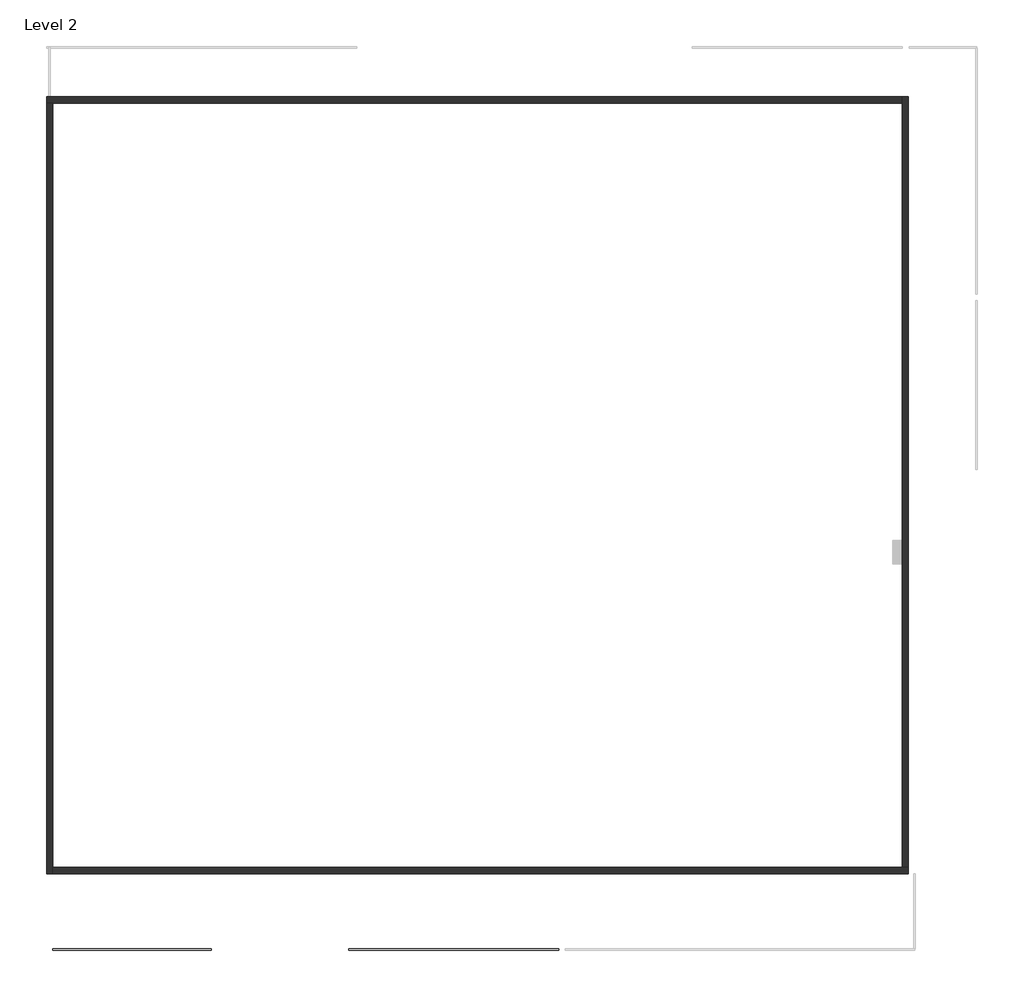
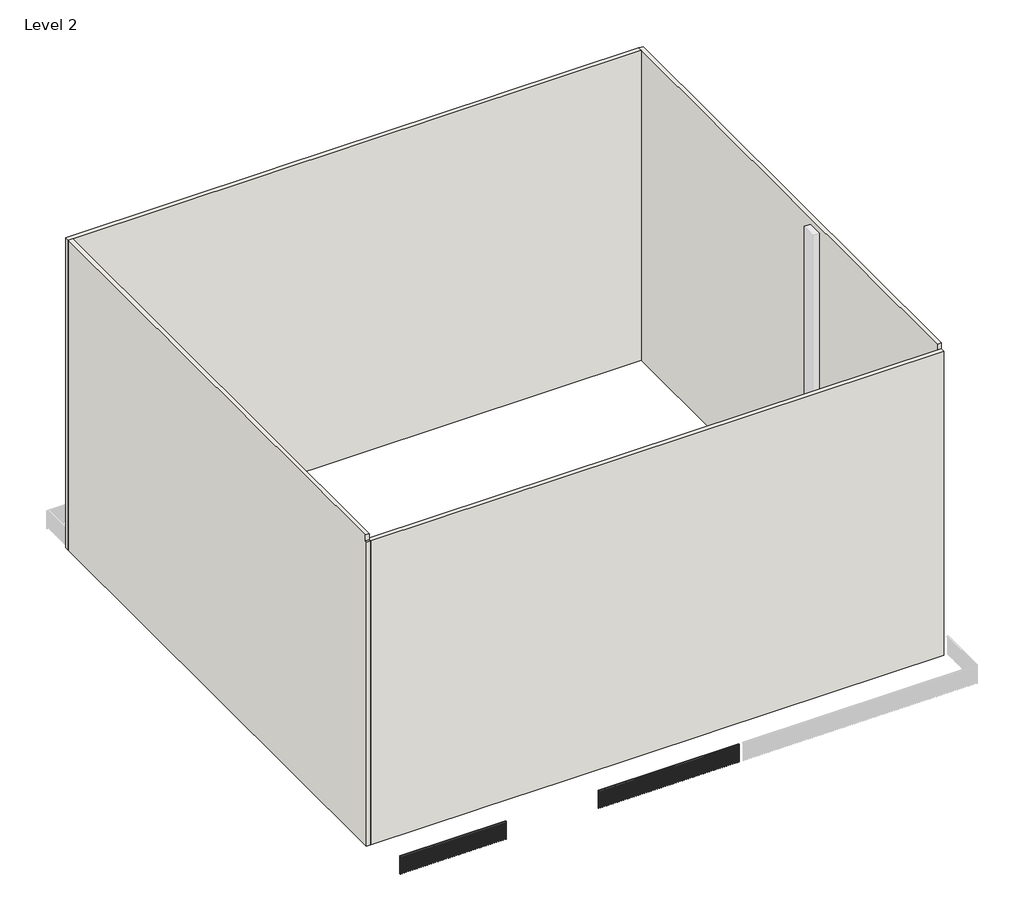
# One storey, part 1 of 5: 4 walls, 2 railings.
"""IFC4 building model written with IfcOpenShell, lengths in millimetres."""

from ifc_helpers import new_model, si_unit, frame, origin, place, context, project, spatial, polyline, outline, extrude, faceted_brep, element, save

model = new_model("IFC4")

# Units and contexts
model_context = context("Model", 3, world=origin())
ifc_project = project(units=[si_unit("LENGTHUNIT", "METRE", prefix="MILLI")], contexts=[model_context])

# Site, building, storey
site = spatial("IfcSite", under=ifc_project)
building = spatial("IfcBuilding", under=site)
storey = spatial("IfcBuildingStorey", under=building, Name="Level 2", Elevation=3048.0)

# Railings
placement = place(None, origin())
element("IfcRailing", 1, ObjectType="Handrail - Rectangular", at=placement, inside=storey, context=model_context, shape_type="SweptSolid", body=[
    extrude(outline(polyline([(-13630.2638778, -12911.7749501), (-13630.2638778, -12860.9749501), (-8499.4638778, -12860.9749501), (-8499.4638778, -12911.7749501), (-13630.2638778, -12911.7749501)])), frame((0.0, 0.0, 3911.6), z_axis=(0.0, 0.0, 1.0), x_axis=(1.0, 0.0, 0.0)), (0.0, 0.0, 1.0), 50.8),
    extrude(outline(polyline([(-8559.7888778, -12895.8999501), (-8559.7888778, -12876.8499501), (-8540.7388778, -12876.8499501), (-8540.7388778, -12895.8999501), (-8559.7888778, -12895.8999501)])), frame((0.0, 0.0, 3048.0), z_axis=(0.0, 0.0, 1.0), x_axis=(1.0, 0.0, 0.0)), (0.0, 0.0, 1.0), 863.6),
    extrude(outline(polyline([(-8661.3888778, -12895.8999501), (-8661.3888778, -12876.8499501), (-8642.3388778, -12876.8499501), (-8642.3388778, -12895.8999501), (-8661.3888778, -12895.8999501)])), frame((0.0, 0.0, 3048.0), z_axis=(0.0, 0.0, 1.0), x_axis=(1.0, 0.0, 0.0)), (0.0, 0.0, 1.0), 863.6),
    extrude(outline(polyline([(-8762.9888778, -12895.8999501), (-8762.9888778, -12876.8499501), (-8743.9388778, -12876.8499501), (-8743.9388778, -12895.8999501), (-8762.9888778, -12895.8999501)])), frame((0.0, 0.0, 3048.0), z_axis=(0.0, 0.0, 1.0), x_axis=(1.0, 0.0, 0.0)), (0.0, 0.0, 1.0), 863.6),
    extrude(outline(polyline([(-8864.5888778, -12895.8999501), (-8864.5888778, -12876.8499501), (-8845.5388778, -12876.8499501), (-8845.5388778, -12895.8999501), (-8864.5888778, -12895.8999501)])), frame((0.0, 0.0, 3048.0), z_axis=(0.0, 0.0, 1.0), x_axis=(1.0, 0.0, 0.0)), (0.0, 0.0, 1.0), 863.6),
    extrude(outline(polyline([(-8966.1888778, -12895.8999501), (-8966.1888778, -12876.8499501), (-8947.1388778, -12876.8499501), (-8947.1388778, -12895.8999501), (-8966.1888778, -12895.8999501)])), frame((0.0, 0.0, 3048.0), z_axis=(0.0, 0.0, 1.0), x_axis=(1.0, 0.0, 0.0)), (0.0, 0.0, 1.0), 863.6),
    extrude(outline(polyline([(-9067.7888778, -12895.8999501), (-9067.7888778, -12876.8499501), (-9048.7388778, -12876.8499501), (-9048.7388778, -12895.8999501), (-9067.7888778, -12895.8999501)])), frame((0.0, 0.0, 3048.0), z_axis=(0.0, 0.0, 1.0), x_axis=(1.0, 0.0, 0.0)), (0.0, 0.0, 1.0), 863.6),
    extrude(outline(polyline([(-9169.3888778, -12895.8999501), (-9169.3888778, -12876.8499501), (-9150.3388778, -12876.8499501), (-9150.3388778, -12895.8999501), (-9169.3888778, -12895.8999501)])), frame((0.0, 0.0, 3048.0), z_axis=(0.0, 0.0, 1.0), x_axis=(1.0, 0.0, 0.0)), (0.0, 0.0, 1.0), 863.6),
    extrude(outline(polyline([(-9270.9888778, -12895.8999501), (-9270.9888778, -12876.8499501), (-9251.9388778, -12876.8499501), (-9251.9388778, -12895.8999501), (-9270.9888778, -12895.8999501)])), frame((0.0, 0.0, 3048.0), z_axis=(0.0, 0.0, 1.0), x_axis=(1.0, 0.0, 0.0)), (0.0, 0.0, 1.0), 863.6),
    extrude(outline(polyline([(-9372.5888778, -12895.8999501), (-9372.5888778, -12876.8499501), (-9353.5388778, -12876.8499501), (-9353.5388778, -12895.8999501), (-9372.5888778, -12895.8999501)])), frame((0.0, 0.0, 3048.0), z_axis=(0.0, 0.0, 1.0), x_axis=(1.0, 0.0, 0.0)), (0.0, 0.0, 1.0), 863.6),
    extrude(outline(polyline([(-9474.1888778, -12895.8999501), (-9474.1888778, -12876.8499501), (-9455.1388778, -12876.8499501), (-9455.1388778, -12895.8999501), (-9474.1888778, -12895.8999501)])), frame((0.0, 0.0, 3048.0), z_axis=(0.0, 0.0, 1.0), x_axis=(1.0, 0.0, 0.0)), (0.0, 0.0, 1.0), 863.6),
    extrude(outline(polyline([(-9575.7888778, -12895.8999501), (-9575.7888778, -12876.8499501), (-9556.7388778, -12876.8499501), (-9556.7388778, -12895.8999501), (-9575.7888778, -12895.8999501)])), frame((0.0, 0.0, 3048.0), z_axis=(0.0, 0.0, 1.0), x_axis=(1.0, 0.0, 0.0)), (0.0, 0.0, 1.0), 863.6),
    extrude(outline(polyline([(-9677.3888778, -12895.8999501), (-9677.3888778, -12876.8499501), (-9658.3388778, -12876.8499501), (-9658.3388778, -12895.8999501), (-9677.3888778, -12895.8999501)])), frame((0.0, 0.0, 3048.0), z_axis=(0.0, 0.0, 1.0), x_axis=(1.0, 0.0, 0.0)), (0.0, 0.0, 1.0), 863.6),
    extrude(outline(polyline([(-9778.9888778, -12895.8999501), (-9778.9888778, -12876.8499501), (-9759.9388778, -12876.8499501), (-9759.9388778, -12895.8999501), (-9778.9888778, -12895.8999501)])), frame((0.0, 0.0, 3048.0), z_axis=(0.0, 0.0, 1.0), x_axis=(1.0, 0.0, 0.0)), (0.0, 0.0, 1.0), 863.6),
    extrude(outline(polyline([(-9880.5888778, -12895.8999501), (-9880.5888778, -12876.8499501), (-9861.5388778, -12876.8499501), (-9861.5388778, -12895.8999501), (-9880.5888778, -12895.8999501)])), frame((0.0, 0.0, 3048.0), z_axis=(0.0, 0.0, 1.0), x_axis=(1.0, 0.0, 0.0)), (0.0, 0.0, 1.0), 863.6),
    extrude(outline(polyline([(-9982.1888778, -12895.8999501), (-9982.1888778, -12876.8499501), (-9963.1388778, -12876.8499501), (-9963.1388778, -12895.8999501), (-9982.1888778, -12895.8999501)])), frame((0.0, 0.0, 3048.0), z_axis=(0.0, 0.0, 1.0), x_axis=(1.0, 0.0, 0.0)), (0.0, 0.0, 1.0), 863.6),
    extrude(outline(polyline([(-10083.7888778, -12895.8999501), (-10083.7888778, -12876.8499501), (-10064.7388778, -12876.8499501), (-10064.7388778, -12895.8999501), (-10083.7888778, -12895.8999501)])), frame((0.0, 0.0, 3048.0), z_axis=(0.0, 0.0, 1.0), x_axis=(1.0, 0.0, 0.0)), (0.0, 0.0, 1.0), 863.6),
    extrude(outline(polyline([(-10185.3888778, -12895.8999501), (-10185.3888778, -12876.8499501), (-10166.3388778, -12876.8499501), (-10166.3388778, -12895.8999501), (-10185.3888778, -12895.8999501)])), frame((0.0, 0.0, 3048.0), z_axis=(0.0, 0.0, 1.0), x_axis=(1.0, 0.0, 0.0)), (0.0, 0.0, 1.0), 863.6),
    extrude(outline(polyline([(-10286.9888778, -12895.8999501), (-10286.9888778, -12876.8499501), (-10267.9388778, -12876.8499501), (-10267.9388778, -12895.8999501), (-10286.9888778, -12895.8999501)])), frame((0.0, 0.0, 3048.0), z_axis=(0.0, 0.0, 1.0), x_axis=(1.0, 0.0, 0.0)), (0.0, 0.0, 1.0), 863.6),
    extrude(outline(polyline([(-10388.5888778, -12895.8999501), (-10388.5888778, -12876.8499501), (-10369.5388778, -12876.8499501), (-10369.5388778, -12895.8999501), (-10388.5888778, -12895.8999501)])), frame((0.0, 0.0, 3048.0), z_axis=(0.0, 0.0, 1.0), x_axis=(1.0, 0.0, 0.0)), (0.0, 0.0, 1.0), 863.6),
    extrude(outline(polyline([(-10490.1888778, -12895.8999501), (-10490.1888778, -12876.8499501), (-10471.1388778, -12876.8499501), (-10471.1388778, -12895.8999501), (-10490.1888778, -12895.8999501)])), frame((0.0, 0.0, 3048.0), z_axis=(0.0, 0.0, 1.0), x_axis=(1.0, 0.0, 0.0)), (0.0, 0.0, 1.0), 863.6),
    extrude(outline(polyline([(-10591.7888778, -12895.8999501), (-10591.7888778, -12876.8499501), (-10572.7388778, -12876.8499501), (-10572.7388778, -12895.8999501), (-10591.7888778, -12895.8999501)])), frame((0.0, 0.0, 3048.0), z_axis=(0.0, 0.0, 1.0), x_axis=(1.0, 0.0, 0.0)), (0.0, 0.0, 1.0), 863.6),
    extrude(outline(polyline([(-10693.3888778, -12895.8999501), (-10693.3888778, -12876.8499501), (-10674.3388778, -12876.8499501), (-10674.3388778, -12895.8999501), (-10693.3888778, -12895.8999501)])), frame((0.0, 0.0, 3048.0), z_axis=(0.0, 0.0, 1.0), x_axis=(1.0, 0.0, 0.0)), (0.0, 0.0, 1.0), 863.6),
    extrude(outline(polyline([(-10794.9888778, -12895.8999501), (-10794.9888778, -12876.8499501), (-10775.9388778, -12876.8499501), (-10775.9388778, -12895.8999501), (-10794.9888778, -12895.8999501)])), frame((0.0, 0.0, 3048.0), z_axis=(0.0, 0.0, 1.0), x_axis=(1.0, 0.0, 0.0)), (0.0, 0.0, 1.0), 863.6),
    extrude(outline(polyline([(-10896.5888778, -12895.8999501), (-10896.5888778, -12876.8499501), (-10877.5388778, -12876.8499501), (-10877.5388778, -12895.8999501), (-10896.5888778, -12895.8999501)])), frame((0.0, 0.0, 3048.0), z_axis=(0.0, 0.0, 1.0), x_axis=(1.0, 0.0, 0.0)), (0.0, 0.0, 1.0), 863.6),
    extrude(outline(polyline([(-10998.1888778, -12895.8999501), (-10998.1888778, -12876.8499501), (-10979.1388778, -12876.8499501), (-10979.1388778, -12895.8999501), (-10998.1888778, -12895.8999501)])), frame((0.0, 0.0, 3048.0), z_axis=(0.0, 0.0, 1.0), x_axis=(1.0, 0.0, 0.0)), (0.0, 0.0, 1.0), 863.6),
    extrude(outline(polyline([(-11099.7888778, -12895.8999501), (-11099.7888778, -12876.8499501), (-11080.7388778, -12876.8499501), (-11080.7388778, -12895.8999501), (-11099.7888778, -12895.8999501)])), frame((0.0, 0.0, 3048.0), z_axis=(0.0, 0.0, 1.0), x_axis=(1.0, 0.0, 0.0)), (0.0, 0.0, 1.0), 863.6),
    extrude(outline(polyline([(-11201.3888778, -12895.8999501), (-11201.3888778, -12876.8499501), (-11182.3388778, -12876.8499501), (-11182.3388778, -12895.8999501), (-11201.3888778, -12895.8999501)])), frame((0.0, 0.0, 3048.0), z_axis=(0.0, 0.0, 1.0), x_axis=(1.0, 0.0, 0.0)), (0.0, 0.0, 1.0), 863.6),
    extrude(outline(polyline([(-11302.9888778, -12895.8999501), (-11302.9888778, -12876.8499501), (-11283.9388778, -12876.8499501), (-11283.9388778, -12895.8999501), (-11302.9888778, -12895.8999501)])), frame((0.0, 0.0, 3048.0), z_axis=(0.0, 0.0, 1.0), x_axis=(1.0, 0.0, 0.0)), (0.0, 0.0, 1.0), 863.6),
    extrude(outline(polyline([(-11404.5888778, -12895.8999501), (-11404.5888778, -12876.8499501), (-11385.5388778, -12876.8499501), (-11385.5388778, -12895.8999501), (-11404.5888778, -12895.8999501)])), frame((0.0, 0.0, 3048.0), z_axis=(0.0, 0.0, 1.0), x_axis=(1.0, 0.0, 0.0)), (0.0, 0.0, 1.0), 863.6),
    extrude(outline(polyline([(-11506.1888778, -12895.8999501), (-11506.1888778, -12876.8499501), (-11487.1388778, -12876.8499501), (-11487.1388778, -12895.8999501), (-11506.1888778, -12895.8999501)])), frame((0.0, 0.0, 3048.0), z_axis=(0.0, 0.0, 1.0), x_axis=(1.0, 0.0, 0.0)), (0.0, 0.0, 1.0), 863.6),
    extrude(outline(polyline([(-11607.7888778, -12895.8999501), (-11607.7888778, -12876.8499501), (-11588.7388778, -12876.8499501), (-11588.7388778, -12895.8999501), (-11607.7888778, -12895.8999501)])), frame((0.0, 0.0, 3048.0), z_axis=(0.0, 0.0, 1.0), x_axis=(1.0, 0.0, 0.0)), (0.0, 0.0, 1.0), 863.6),
    extrude(outline(polyline([(-11709.3888778, -12895.8999501), (-11709.3888778, -12876.8499501), (-11690.3388778, -12876.8499501), (-11690.3388778, -12895.8999501), (-11709.3888778, -12895.8999501)])), frame((0.0, 0.0, 3048.0), z_axis=(0.0, 0.0, 1.0), x_axis=(1.0, 0.0, 0.0)), (0.0, 0.0, 1.0), 863.6),
    extrude(outline(polyline([(-11810.9888778, -12895.8999501), (-11810.9888778, -12876.8499501), (-11791.9388778, -12876.8499501), (-11791.9388778, -12895.8999501), (-11810.9888778, -12895.8999501)])), frame((0.0, 0.0, 3048.0), z_axis=(0.0, 0.0, 1.0), x_axis=(1.0, 0.0, 0.0)), (0.0, 0.0, 1.0), 863.6),
    extrude(outline(polyline([(-11912.5888778, -12895.8999501), (-11912.5888778, -12876.8499501), (-11893.5388778, -12876.8499501), (-11893.5388778, -12895.8999501), (-11912.5888778, -12895.8999501)])), frame((0.0, 0.0, 3048.0), z_axis=(0.0, 0.0, 1.0), x_axis=(1.0, 0.0, 0.0)), (0.0, 0.0, 1.0), 863.6),
    extrude(outline(polyline([(-12014.1888778, -12895.8999501), (-12014.1888778, -12876.8499501), (-11995.1388778, -12876.8499501), (-11995.1388778, -12895.8999501), (-12014.1888778, -12895.8999501)])), frame((0.0, 0.0, 3048.0), z_axis=(0.0, 0.0, 1.0), x_axis=(1.0, 0.0, 0.0)), (0.0, 0.0, 1.0), 863.6),
    extrude(outline(polyline([(-12115.7888778, -12895.8999501), (-12115.7888778, -12876.8499501), (-12096.7388778, -12876.8499501), (-12096.7388778, -12895.8999501), (-12115.7888778, -12895.8999501)])), frame((0.0, 0.0, 3048.0), z_axis=(0.0, 0.0, 1.0), x_axis=(1.0, 0.0, 0.0)), (0.0, 0.0, 1.0), 863.6),
    extrude(outline(polyline([(-12217.3888778, -12895.8999501), (-12217.3888778, -12876.8499501), (-12198.3388778, -12876.8499501), (-12198.3388778, -12895.8999501), (-12217.3888778, -12895.8999501)])), frame((0.0, 0.0, 3048.0), z_axis=(0.0, 0.0, 1.0), x_axis=(1.0, 0.0, 0.0)), (0.0, 0.0, 1.0), 863.6),
    extrude(outline(polyline([(-12318.9888778, -12895.8999501), (-12318.9888778, -12876.8499501), (-12299.9388778, -12876.8499501), (-12299.9388778, -12895.8999501), (-12318.9888778, -12895.8999501)])), frame((0.0, 0.0, 3048.0), z_axis=(0.0, 0.0, 1.0), x_axis=(1.0, 0.0, 0.0)), (0.0, 0.0, 1.0), 863.6),
    extrude(outline(polyline([(-12420.5888778, -12895.8999501), (-12420.5888778, -12876.8499501), (-12401.5388778, -12876.8499501), (-12401.5388778, -12895.8999501), (-12420.5888778, -12895.8999501)])), frame((0.0, 0.0, 3048.0), z_axis=(0.0, 0.0, 1.0), x_axis=(1.0, 0.0, 0.0)), (0.0, 0.0, 1.0), 863.6),
    extrude(outline(polyline([(-12522.1888778, -12895.8999501), (-12522.1888778, -12876.8499501), (-12503.1388778, -12876.8499501), (-12503.1388778, -12895.8999501), (-12522.1888778, -12895.8999501)])), frame((0.0, 0.0, 3048.0), z_axis=(0.0, 0.0, 1.0), x_axis=(1.0, 0.0, 0.0)), (0.0, 0.0, 1.0), 863.6),
    extrude(outline(polyline([(-12623.7888778, -12895.8999501), (-12623.7888778, -12876.8499501), (-12604.7388778, -12876.8499501), (-12604.7388778, -12895.8999501), (-12623.7888778, -12895.8999501)])), frame((0.0, 0.0, 3048.0), z_axis=(0.0, 0.0, 1.0), x_axis=(1.0, 0.0, 0.0)), (0.0, 0.0, 1.0), 863.6),
    extrude(outline(polyline([(-12725.3888778, -12895.8999501), (-12725.3888778, -12876.8499501), (-12706.3388778, -12876.8499501), (-12706.3388778, -12895.8999501), (-12725.3888778, -12895.8999501)])), frame((0.0, 0.0, 3048.0), z_axis=(0.0, 0.0, 1.0), x_axis=(1.0, 0.0, 0.0)), (0.0, 0.0, 1.0), 863.6),
    extrude(outline(polyline([(-12826.9888778, -12895.8999501), (-12826.9888778, -12876.8499501), (-12807.9388778, -12876.8499501), (-12807.9388778, -12895.8999501), (-12826.9888778, -12895.8999501)])), frame((0.0, 0.0, 3048.0), z_axis=(0.0, 0.0, 1.0), x_axis=(1.0, 0.0, 0.0)), (0.0, 0.0, 1.0), 863.6),
    extrude(outline(polyline([(-12928.5888778, -12895.8999501), (-12928.5888778, -12876.8499501), (-12909.5388778, -12876.8499501), (-12909.5388778, -12895.8999501), (-12928.5888778, -12895.8999501)])), frame((0.0, 0.0, 3048.0), z_axis=(0.0, 0.0, 1.0), x_axis=(1.0, 0.0, 0.0)), (0.0, 0.0, 1.0), 863.6),
    extrude(outline(polyline([(-13030.1888778, -12895.8999501), (-13030.1888778, -12876.8499501), (-13011.1388778, -12876.8499501), (-13011.1388778, -12895.8999501), (-13030.1888778, -12895.8999501)])), frame((0.0, 0.0, 3048.0), z_axis=(0.0, 0.0, 1.0), x_axis=(1.0, 0.0, 0.0)), (0.0, 0.0, 1.0), 863.6),
    extrude(outline(polyline([(-13131.7888778, -12895.8999501), (-13131.7888778, -12876.8499501), (-13112.7388778, -12876.8499501), (-13112.7388778, -12895.8999501), (-13131.7888778, -12895.8999501)])), frame((0.0, 0.0, 3048.0), z_axis=(0.0, 0.0, 1.0), x_axis=(1.0, 0.0, 0.0)), (0.0, 0.0, 1.0), 863.6),
    extrude(outline(polyline([(-13233.3888778, -12895.8999501), (-13233.3888778, -12876.8499501), (-13214.3388778, -12876.8499501), (-13214.3388778, -12895.8999501), (-13233.3888778, -12895.8999501)])), frame((0.0, 0.0, 3048.0), z_axis=(0.0, 0.0, 1.0), x_axis=(1.0, 0.0, 0.0)), (0.0, 0.0, 1.0), 863.6),
    extrude(outline(polyline([(-13334.9888778, -12895.8999501), (-13334.9888778, -12876.8499501), (-13315.9388778, -12876.8499501), (-13315.9388778, -12895.8999501), (-13334.9888778, -12895.8999501)])), frame((0.0, 0.0, 3048.0), z_axis=(0.0, 0.0, 1.0), x_axis=(1.0, 0.0, 0.0)), (0.0, 0.0, 1.0), 863.6),
    extrude(outline(polyline([(-13436.5888778, -12895.8999501), (-13436.5888778, -12876.8499501), (-13417.5388778, -12876.8499501), (-13417.5388778, -12895.8999501), (-13436.5888778, -12895.8999501)])), frame((0.0, 0.0, 3048.0), z_axis=(0.0, 0.0, 1.0), x_axis=(1.0, 0.0, 0.0)), (0.0, 0.0, 1.0), 863.6),
    extrude(outline(polyline([(-13538.1888778, -12895.8999501), (-13538.1888778, -12876.8499501), (-13519.1388778, -12876.8499501), (-13519.1388778, -12895.8999501), (-13538.1888778, -12895.8999501)])), frame((0.0, 0.0, 3048.0), z_axis=(0.0, 0.0, 1.0), x_axis=(1.0, 0.0, 0.0)), (0.0, 0.0, 1.0), 863.6),
    extrude(outline(polyline([(-8518.5138778, -12895.8999501), (-8518.5138778, -12876.8499501), (-8499.4638778, -12876.8499501), (-8499.4638778, -12895.8999501), (-8518.5138778, -12895.8999501)])), frame((0.0, 0.0, 3048.0), z_axis=(0.0, 0.0, 1.0), x_axis=(1.0, 0.0, 0.0)), (0.0, 0.0, 1.0), 863.6),
    extrude(outline(polyline([(-13630.2638778, -12895.8999501), (-13630.2638778, -12876.8499501), (-13611.2138778, -12876.8499501), (-13611.2138778, -12895.8999501), (-13630.2638778, -12895.8999501)])), frame((0.0, 0.0, 3048.0), z_axis=(0.0, 0.0, 1.0), x_axis=(1.0, 0.0, 0.0)), (0.0, 0.0, 1.0), 863.6),
])
element("IfcRailing", 2, ObjectType="Handrail - Rectangular", at=placement, inside=storey, context=model_context, shape_type="SweptSolid", body=[
    extrude(outline(polyline([(-4029.0638778, -12911.7749501), (-4029.0638778, -12860.9749501), (2778.1361222, -12860.9749501), (2778.1361222, -12911.7749501), (-4029.0638778, -12911.7749501)])), frame((0.0, 0.0, 3911.6), z_axis=(0.0, 0.0, 1.0), x_axis=(1.0, 0.0, 0.0)), (0.0, 0.0, 1.0), 50.8),
    extrude(outline(polyline([(2667.0111222, -12895.8999501), (2667.0111222, -12876.8499501), (2686.0611222, -12876.8499501), (2686.0611222, -12895.8999501), (2667.0111222, -12895.8999501)])), frame((0.0, 0.0, 3048.0), z_axis=(0.0, 0.0, 1.0), x_axis=(1.0, 0.0, 0.0)), (0.0, 0.0, 1.0), 863.6),
    extrude(outline(polyline([(2565.4111222, -12895.8999501), (2565.4111222, -12876.8499501), (2584.4611222, -12876.8499501), (2584.4611222, -12895.8999501), (2565.4111222, -12895.8999501)])), frame((0.0, 0.0, 3048.0), z_axis=(0.0, 0.0, 1.0), x_axis=(1.0, 0.0, 0.0)), (0.0, 0.0, 1.0), 863.6),
    extrude(outline(polyline([(2463.8111222, -12895.8999501), (2463.8111222, -12876.8499501), (2482.8611222, -12876.8499501), (2482.8611222, -12895.8999501), (2463.8111222, -12895.8999501)])), frame((0.0, 0.0, 3048.0), z_axis=(0.0, 0.0, 1.0), x_axis=(1.0, 0.0, 0.0)), (0.0, 0.0, 1.0), 863.6),
    extrude(outline(polyline([(2362.2111222, -12895.8999501), (2362.2111222, -12876.8499501), (2381.2611222, -12876.8499501), (2381.2611222, -12895.8999501), (2362.2111222, -12895.8999501)])), frame((0.0, 0.0, 3048.0), z_axis=(0.0, 0.0, 1.0), x_axis=(1.0, 0.0, 0.0)), (0.0, 0.0, 1.0), 863.6),
    extrude(outline(polyline([(2260.6111222, -12895.8999501), (2260.6111222, -12876.8499501), (2279.6611222, -12876.8499501), (2279.6611222, -12895.8999501), (2260.6111222, -12895.8999501)])), frame((0.0, 0.0, 3048.0), z_axis=(0.0, 0.0, 1.0), x_axis=(1.0, 0.0, 0.0)), (0.0, 0.0, 1.0), 863.6),
    extrude(outline(polyline([(2159.0111222, -12895.8999501), (2159.0111222, -12876.8499501), (2178.0611222, -12876.8499501), (2178.0611222, -12895.8999501), (2159.0111222, -12895.8999501)])), frame((0.0, 0.0, 3048.0), z_axis=(0.0, 0.0, 1.0), x_axis=(1.0, 0.0, 0.0)), (0.0, 0.0, 1.0), 863.6),
    extrude(outline(polyline([(2057.4111222, -12895.8999501), (2057.4111222, -12876.8499501), (2076.4611222, -12876.8499501), (2076.4611222, -12895.8999501), (2057.4111222, -12895.8999501)])), frame((0.0, 0.0, 3048.0), z_axis=(0.0, 0.0, 1.0), x_axis=(1.0, 0.0, 0.0)), (0.0, 0.0, 1.0), 863.6),
    extrude(outline(polyline([(1955.8111222, -12895.8999501), (1955.8111222, -12876.8499501), (1974.8611222, -12876.8499501), (1974.8611222, -12895.8999501), (1955.8111222, -12895.8999501)])), frame((0.0, 0.0, 3048.0), z_axis=(0.0, 0.0, 1.0), x_axis=(1.0, 0.0, 0.0)), (0.0, 0.0, 1.0), 863.6),
    extrude(outline(polyline([(1854.2111222, -12895.8999501), (1854.2111222, -12876.8499501), (1873.2611222, -12876.8499501), (1873.2611222, -12895.8999501), (1854.2111222, -12895.8999501)])), frame((0.0, 0.0, 3048.0), z_axis=(0.0, 0.0, 1.0), x_axis=(1.0, 0.0, 0.0)), (0.0, 0.0, 1.0), 863.6),
    extrude(outline(polyline([(1752.6111222, -12895.8999501), (1752.6111222, -12876.8499501), (1771.6611222, -12876.8499501), (1771.6611222, -12895.8999501), (1752.6111222, -12895.8999501)])), frame((0.0, 0.0, 3048.0), z_axis=(0.0, 0.0, 1.0), x_axis=(1.0, 0.0, 0.0)), (0.0, 0.0, 1.0), 863.6),
    extrude(outline(polyline([(1651.0111222, -12895.8999501), (1651.0111222, -12876.8499501), (1670.0611222, -12876.8499501), (1670.0611222, -12895.8999501), (1651.0111222, -12895.8999501)])), frame((0.0, 0.0, 3048.0), z_axis=(0.0, 0.0, 1.0), x_axis=(1.0, 0.0, 0.0)), (0.0, 0.0, 1.0), 863.6),
    extrude(outline(polyline([(1549.4111222, -12895.8999501), (1549.4111222, -12876.8499501), (1568.4611222, -12876.8499501), (1568.4611222, -12895.8999501), (1549.4111222, -12895.8999501)])), frame((0.0, 0.0, 3048.0), z_axis=(0.0, 0.0, 1.0), x_axis=(1.0, 0.0, 0.0)), (0.0, 0.0, 1.0), 863.6),
    extrude(outline(polyline([(1447.8111222, -12895.8999501), (1447.8111222, -12876.8499501), (1466.8611222, -12876.8499501), (1466.8611222, -12895.8999501), (1447.8111222, -12895.8999501)])), frame((0.0, 0.0, 3048.0), z_axis=(0.0, 0.0, 1.0), x_axis=(1.0, 0.0, 0.0)), (0.0, 0.0, 1.0), 863.6),
    extrude(outline(polyline([(1346.2111222, -12895.8999501), (1346.2111222, -12876.8499501), (1365.2611222, -12876.8499501), (1365.2611222, -12895.8999501), (1346.2111222, -12895.8999501)])), frame((0.0, 0.0, 3048.0), z_axis=(0.0, 0.0, 1.0), x_axis=(1.0, 0.0, 0.0)), (0.0, 0.0, 1.0), 863.6),
    extrude(outline(polyline([(1244.6111222, -12895.8999501), (1244.6111222, -12876.8499501), (1263.6611222, -12876.8499501), (1263.6611222, -12895.8999501), (1244.6111222, -12895.8999501)])), frame((0.0, 0.0, 3048.0), z_axis=(0.0, 0.0, 1.0), x_axis=(1.0, 0.0, 0.0)), (0.0, 0.0, 1.0), 863.6),
    extrude(outline(polyline([(1143.0111222, -12895.8999501), (1143.0111222, -12876.8499501), (1162.0611222, -12876.8499501), (1162.0611222, -12895.8999501), (1143.0111222, -12895.8999501)])), frame((0.0, 0.0, 3048.0), z_axis=(0.0, 0.0, 1.0), x_axis=(1.0, 0.0, 0.0)), (0.0, 0.0, 1.0), 863.6),
    extrude(outline(polyline([(1041.4111222, -12895.8999501), (1041.4111222, -12876.8499501), (1060.4611222, -12876.8499501), (1060.4611222, -12895.8999501), (1041.4111222, -12895.8999501)])), frame((0.0, 0.0, 3048.0), z_axis=(0.0, 0.0, 1.0), x_axis=(1.0, 0.0, 0.0)), (0.0, 0.0, 1.0), 863.6),
    extrude(outline(polyline([(939.8111222, -12895.8999501), (939.8111222, -12876.8499501), (958.8611222, -12876.8499501), (958.8611222, -12895.8999501), (939.8111222, -12895.8999501)])), frame((0.0, 0.0, 3048.0), z_axis=(0.0, 0.0, 1.0), x_axis=(1.0, 0.0, 0.0)), (0.0, 0.0, 1.0), 863.6),
    extrude(outline(polyline([(838.2111222, -12895.8999501), (838.2111222, -12876.8499501), (857.2611222, -12876.8499501), (857.2611222, -12895.8999501), (838.2111222, -12895.8999501)])), frame((0.0, 0.0, 3048.0), z_axis=(0.0, 0.0, 1.0), x_axis=(1.0, 0.0, 0.0)), (0.0, 0.0, 1.0), 863.6),
    extrude(outline(polyline([(736.6111222, -12895.8999501), (736.6111222, -12876.8499501), (755.6611222, -12876.8499501), (755.6611222, -12895.8999501), (736.6111222, -12895.8999501)])), frame((0.0, 0.0, 3048.0), z_axis=(0.0, 0.0, 1.0), x_axis=(1.0, 0.0, 0.0)), (0.0, 0.0, 1.0), 863.6),
    extrude(outline(polyline([(635.0111222, -12895.8999501), (635.0111222, -12876.8499501), (654.0611222, -12876.8499501), (654.0611222, -12895.8999501), (635.0111222, -12895.8999501)])), frame((0.0, 0.0, 3048.0), z_axis=(0.0, 0.0, 1.0), x_axis=(1.0, 0.0, 0.0)), (0.0, 0.0, 1.0), 863.6),
    extrude(outline(polyline([(533.4111222, -12895.8999501), (533.4111222, -12876.8499501), (552.4611222, -12876.8499501), (552.4611222, -12895.8999501), (533.4111222, -12895.8999501)])), frame((0.0, 0.0, 3048.0), z_axis=(0.0, 0.0, 1.0), x_axis=(1.0, 0.0, 0.0)), (0.0, 0.0, 1.0), 863.6),
    extrude(outline(polyline([(431.8111222, -12895.8999501), (431.8111222, -12876.8499501), (450.8611222, -12876.8499501), (450.8611222, -12895.8999501), (431.8111222, -12895.8999501)])), frame((0.0, 0.0, 3048.0), z_axis=(0.0, 0.0, 1.0), x_axis=(1.0, 0.0, 0.0)), (0.0, 0.0, 1.0), 863.6),
    extrude(outline(polyline([(330.2111222, -12895.8999501), (330.2111222, -12876.8499501), (349.2611222, -12876.8499501), (349.2611222, -12895.8999501), (330.2111222, -12895.8999501)])), frame((0.0, 0.0, 3048.0), z_axis=(0.0, 0.0, 1.0), x_axis=(1.0, 0.0, 0.0)), (0.0, 0.0, 1.0), 863.6),
    extrude(outline(polyline([(228.6111222, -12895.8999501), (228.6111222, -12876.8499501), (247.6611222, -12876.8499501), (247.6611222, -12895.8999501), (228.6111222, -12895.8999501)])), frame((0.0, 0.0, 3048.0), z_axis=(0.0, 0.0, 1.0), x_axis=(1.0, 0.0, 0.0)), (0.0, 0.0, 1.0), 863.6),
    extrude(outline(polyline([(127.0111222, -12895.8999501), (127.0111222, -12876.8499501), (146.0611222, -12876.8499501), (146.0611222, -12895.8999501), (127.0111222, -12895.8999501)])), frame((0.0, 0.0, 3048.0), z_axis=(0.0, 0.0, 1.0), x_axis=(1.0, 0.0, 0.0)), (0.0, 0.0, 1.0), 863.6),
    extrude(outline(polyline([(25.4111222, -12895.8999501), (25.4111222, -12876.8499501), (44.4611222, -12876.8499501), (44.4611222, -12895.8999501), (25.4111222, -12895.8999501)])), frame((0.0, 0.0, 3048.0), z_axis=(0.0, 0.0, 1.0), x_axis=(1.0, 0.0, 0.0)), (0.0, 0.0, 1.0), 863.6),
    extrude(outline(polyline([(-76.1888778, -12895.8999501), (-76.1888778, -12876.8499501), (-57.1388778, -12876.8499501), (-57.1388778, -12895.8999501), (-76.1888778, -12895.8999501)])), frame((0.0, 0.0, 3048.0), z_axis=(0.0, 0.0, 1.0), x_axis=(1.0, 0.0, 0.0)), (0.0, 0.0, 1.0), 863.6),
    extrude(outline(polyline([(-177.7888778, -12895.8999501), (-177.7888778, -12876.8499501), (-158.7388778, -12876.8499501), (-158.7388778, -12895.8999501), (-177.7888778, -12895.8999501)])), frame((0.0, 0.0, 3048.0), z_axis=(0.0, 0.0, 1.0), x_axis=(1.0, 0.0, 0.0)), (0.0, 0.0, 1.0), 863.6),
    extrude(outline(polyline([(-279.3888778, -12895.8999501), (-279.3888778, -12876.8499501), (-260.3388778, -12876.8499501), (-260.3388778, -12895.8999501), (-279.3888778, -12895.8999501)])), frame((0.0, 0.0, 3048.0), z_axis=(0.0, 0.0, 1.0), x_axis=(1.0, 0.0, 0.0)), (0.0, 0.0, 1.0), 863.6),
    extrude(outline(polyline([(-380.9888778, -12895.8999501), (-380.9888778, -12876.8499501), (-361.9388778, -12876.8499501), (-361.9388778, -12895.8999501), (-380.9888778, -12895.8999501)])), frame((0.0, 0.0, 3048.0), z_axis=(0.0, 0.0, 1.0), x_axis=(1.0, 0.0, 0.0)), (0.0, 0.0, 1.0), 863.6),
    extrude(outline(polyline([(-482.5888778, -12895.8999501), (-482.5888778, -12876.8499501), (-463.5388778, -12876.8499501), (-463.5388778, -12895.8999501), (-482.5888778, -12895.8999501)])), frame((0.0, 0.0, 3048.0), z_axis=(0.0, 0.0, 1.0), x_axis=(1.0, 0.0, 0.0)), (0.0, 0.0, 1.0), 863.6),
    extrude(outline(polyline([(-584.1888778, -12895.8999501), (-584.1888778, -12876.8499501), (-565.1388778, -12876.8499501), (-565.1388778, -12895.8999501), (-584.1888778, -12895.8999501)])), frame((0.0, 0.0, 3048.0), z_axis=(0.0, 0.0, 1.0), x_axis=(1.0, 0.0, 0.0)), (0.0, 0.0, 1.0), 863.6),
    extrude(outline(polyline([(-685.7888778, -12895.8999501), (-685.7888778, -12876.8499501), (-666.7388778, -12876.8499501), (-666.7388778, -12895.8999501), (-685.7888778, -12895.8999501)])), frame((0.0, 0.0, 3048.0), z_axis=(0.0, 0.0, 1.0), x_axis=(1.0, 0.0, 0.0)), (0.0, 0.0, 1.0), 863.6),
    extrude(outline(polyline([(-787.3888778, -12895.8999501), (-787.3888778, -12876.8499501), (-768.3388778, -12876.8499501), (-768.3388778, -12895.8999501), (-787.3888778, -12895.8999501)])), frame((0.0, 0.0, 3048.0), z_axis=(0.0, 0.0, 1.0), x_axis=(1.0, 0.0, 0.0)), (0.0, 0.0, 1.0), 863.6),
    extrude(outline(polyline([(-888.9888778, -12895.8999501), (-888.9888778, -12876.8499501), (-869.9388778, -12876.8499501), (-869.9388778, -12895.8999501), (-888.9888778, -12895.8999501)])), frame((0.0, 0.0, 3048.0), z_axis=(0.0, 0.0, 1.0), x_axis=(1.0, 0.0, 0.0)), (0.0, 0.0, 1.0), 863.6),
    extrude(outline(polyline([(-990.5888778, -12895.8999501), (-990.5888778, -12876.8499501), (-971.5388778, -12876.8499501), (-971.5388778, -12895.8999501), (-990.5888778, -12895.8999501)])), frame((0.0, 0.0, 3048.0), z_axis=(0.0, 0.0, 1.0), x_axis=(1.0, 0.0, 0.0)), (0.0, 0.0, 1.0), 863.6),
    extrude(outline(polyline([(-1092.1888778, -12895.8999501), (-1092.1888778, -12876.8499501), (-1073.1388778, -12876.8499501), (-1073.1388778, -12895.8999501), (-1092.1888778, -12895.8999501)])), frame((0.0, 0.0, 3048.0), z_axis=(0.0, 0.0, 1.0), x_axis=(1.0, 0.0, 0.0)), (0.0, 0.0, 1.0), 863.6),
    extrude(outline(polyline([(-1193.7888778, -12895.8999501), (-1193.7888778, -12876.8499501), (-1174.7388778, -12876.8499501), (-1174.7388778, -12895.8999501), (-1193.7888778, -12895.8999501)])), frame((0.0, 0.0, 3048.0), z_axis=(0.0, 0.0, 1.0), x_axis=(1.0, 0.0, 0.0)), (0.0, 0.0, 1.0), 863.6),
    extrude(outline(polyline([(-1295.3888778, -12895.8999501), (-1295.3888778, -12876.8499501), (-1276.3388778, -12876.8499501), (-1276.3388778, -12895.8999501), (-1295.3888778, -12895.8999501)])), frame((0.0, 0.0, 3048.0), z_axis=(0.0, 0.0, 1.0), x_axis=(1.0, 0.0, 0.0)), (0.0, 0.0, 1.0), 863.6),
    extrude(outline(polyline([(-1396.9888778, -12895.8999501), (-1396.9888778, -12876.8499501), (-1377.9388778, -12876.8499501), (-1377.9388778, -12895.8999501), (-1396.9888778, -12895.8999501)])), frame((0.0, 0.0, 3048.0), z_axis=(0.0, 0.0, 1.0), x_axis=(1.0, 0.0, 0.0)), (0.0, 0.0, 1.0), 863.6),
    extrude(outline(polyline([(-1498.5888778, -12895.8999501), (-1498.5888778, -12876.8499501), (-1479.5388778, -12876.8499501), (-1479.5388778, -12895.8999501), (-1498.5888778, -12895.8999501)])), frame((0.0, 0.0, 3048.0), z_axis=(0.0, 0.0, 1.0), x_axis=(1.0, 0.0, 0.0)), (0.0, 0.0, 1.0), 863.6),
    extrude(outline(polyline([(-1600.1888778, -12895.8999501), (-1600.1888778, -12876.8499501), (-1581.1388778, -12876.8499501), (-1581.1388778, -12895.8999501), (-1600.1888778, -12895.8999501)])), frame((0.0, 0.0, 3048.0), z_axis=(0.0, 0.0, 1.0), x_axis=(1.0, 0.0, 0.0)), (0.0, 0.0, 1.0), 863.6),
    extrude(outline(polyline([(-1701.7888778, -12895.8999501), (-1701.7888778, -12876.8499501), (-1682.7388778, -12876.8499501), (-1682.7388778, -12895.8999501), (-1701.7888778, -12895.8999501)])), frame((0.0, 0.0, 3048.0), z_axis=(0.0, 0.0, 1.0), x_axis=(1.0, 0.0, 0.0)), (0.0, 0.0, 1.0), 863.6),
    extrude(outline(polyline([(-1803.3888778, -12895.8999501), (-1803.3888778, -12876.8499501), (-1784.3388778, -12876.8499501), (-1784.3388778, -12895.8999501), (-1803.3888778, -12895.8999501)])), frame((0.0, 0.0, 3048.0), z_axis=(0.0, 0.0, 1.0), x_axis=(1.0, 0.0, 0.0)), (0.0, 0.0, 1.0), 863.6),
    extrude(outline(polyline([(-1904.9888778, -12895.8999501), (-1904.9888778, -12876.8499501), (-1885.9388778, -12876.8499501), (-1885.9388778, -12895.8999501), (-1904.9888778, -12895.8999501)])), frame((0.0, 0.0, 3048.0), z_axis=(0.0, 0.0, 1.0), x_axis=(1.0, 0.0, 0.0)), (0.0, 0.0, 1.0), 863.6),
    extrude(outline(polyline([(-2006.5888778, -12895.8999501), (-2006.5888778, -12876.8499501), (-1987.5388778, -12876.8499501), (-1987.5388778, -12895.8999501), (-2006.5888778, -12895.8999501)])), frame((0.0, 0.0, 3048.0), z_axis=(0.0, 0.0, 1.0), x_axis=(1.0, 0.0, 0.0)), (0.0, 0.0, 1.0), 863.6),
    extrude(outline(polyline([(-2108.1888778, -12895.8999501), (-2108.1888778, -12876.8499501), (-2089.1388778, -12876.8499501), (-2089.1388778, -12895.8999501), (-2108.1888778, -12895.8999501)])), frame((0.0, 0.0, 3048.0), z_axis=(0.0, 0.0, 1.0), x_axis=(1.0, 0.0, 0.0)), (0.0, 0.0, 1.0), 863.6),
    extrude(outline(polyline([(-2209.7888778, -12895.8999501), (-2209.7888778, -12876.8499501), (-2190.7388778, -12876.8499501), (-2190.7388778, -12895.8999501), (-2209.7888778, -12895.8999501)])), frame((0.0, 0.0, 3048.0), z_axis=(0.0, 0.0, 1.0), x_axis=(1.0, 0.0, 0.0)), (0.0, 0.0, 1.0), 863.6),
    extrude(outline(polyline([(-2311.3888778, -12895.8999501), (-2311.3888778, -12876.8499501), (-2292.3388778, -12876.8499501), (-2292.3388778, -12895.8999501), (-2311.3888778, -12895.8999501)])), frame((0.0, 0.0, 3048.0), z_axis=(0.0, 0.0, 1.0), x_axis=(1.0, 0.0, 0.0)), (0.0, 0.0, 1.0), 863.6),
    extrude(outline(polyline([(-2412.9888778, -12895.8999501), (-2412.9888778, -12876.8499501), (-2393.9388778, -12876.8499501), (-2393.9388778, -12895.8999501), (-2412.9888778, -12895.8999501)])), frame((0.0, 0.0, 3048.0), z_axis=(0.0, 0.0, 1.0), x_axis=(1.0, 0.0, 0.0)), (0.0, 0.0, 1.0), 863.6),
    extrude(outline(polyline([(-2514.5888778, -12895.8999501), (-2514.5888778, -12876.8499501), (-2495.5388778, -12876.8499501), (-2495.5388778, -12895.8999501), (-2514.5888778, -12895.8999501)])), frame((0.0, 0.0, 3048.0), z_axis=(0.0, 0.0, 1.0), x_axis=(1.0, 0.0, 0.0)), (0.0, 0.0, 1.0), 863.6),
    extrude(outline(polyline([(-2616.1888778, -12895.8999501), (-2616.1888778, -12876.8499501), (-2597.1388778, -12876.8499501), (-2597.1388778, -12895.8999501), (-2616.1888778, -12895.8999501)])), frame((0.0, 0.0, 3048.0), z_axis=(0.0, 0.0, 1.0), x_axis=(1.0, 0.0, 0.0)), (0.0, 0.0, 1.0), 863.6),
    extrude(outline(polyline([(-2717.7888778, -12895.8999501), (-2717.7888778, -12876.8499501), (-2698.7388778, -12876.8499501), (-2698.7388778, -12895.8999501), (-2717.7888778, -12895.8999501)])), frame((0.0, 0.0, 3048.0), z_axis=(0.0, 0.0, 1.0), x_axis=(1.0, 0.0, 0.0)), (0.0, 0.0, 1.0), 863.6),
    extrude(outline(polyline([(-2819.3888778, -12895.8999501), (-2819.3888778, -12876.8499501), (-2800.3388778, -12876.8499501), (-2800.3388778, -12895.8999501), (-2819.3888778, -12895.8999501)])), frame((0.0, 0.0, 3048.0), z_axis=(0.0, 0.0, 1.0), x_axis=(1.0, 0.0, 0.0)), (0.0, 0.0, 1.0), 863.6),
    extrude(outline(polyline([(-2920.9888778, -12895.8999501), (-2920.9888778, -12876.8499501), (-2901.9388778, -12876.8499501), (-2901.9388778, -12895.8999501), (-2920.9888778, -12895.8999501)])), frame((0.0, 0.0, 3048.0), z_axis=(0.0, 0.0, 1.0), x_axis=(1.0, 0.0, 0.0)), (0.0, 0.0, 1.0), 863.6),
    extrude(outline(polyline([(-3022.5888778, -12895.8999501), (-3022.5888778, -12876.8499501), (-3003.5388778, -12876.8499501), (-3003.5388778, -12895.8999501), (-3022.5888778, -12895.8999501)])), frame((0.0, 0.0, 3048.0), z_axis=(0.0, 0.0, 1.0), x_axis=(1.0, 0.0, 0.0)), (0.0, 0.0, 1.0), 863.6),
    extrude(outline(polyline([(-3124.1888778, -12895.8999501), (-3124.1888778, -12876.8499501), (-3105.1388778, -12876.8499501), (-3105.1388778, -12895.8999501), (-3124.1888778, -12895.8999501)])), frame((0.0, 0.0, 3048.0), z_axis=(0.0, 0.0, 1.0), x_axis=(1.0, 0.0, 0.0)), (0.0, 0.0, 1.0), 863.6),
    extrude(outline(polyline([(-3225.7888778, -12895.8999501), (-3225.7888778, -12876.8499501), (-3206.7388778, -12876.8499501), (-3206.7388778, -12895.8999501), (-3225.7888778, -12895.8999501)])), frame((0.0, 0.0, 3048.0), z_axis=(0.0, 0.0, 1.0), x_axis=(1.0, 0.0, 0.0)), (0.0, 0.0, 1.0), 863.6),
    extrude(outline(polyline([(-3327.3888778, -12895.8999501), (-3327.3888778, -12876.8499501), (-3308.3388778, -12876.8499501), (-3308.3388778, -12895.8999501), (-3327.3888778, -12895.8999501)])), frame((0.0, 0.0, 3048.0), z_axis=(0.0, 0.0, 1.0), x_axis=(1.0, 0.0, 0.0)), (0.0, 0.0, 1.0), 863.6),
    extrude(outline(polyline([(-3428.9888778, -12895.8999501), (-3428.9888778, -12876.8499501), (-3409.9388778, -12876.8499501), (-3409.9388778, -12895.8999501), (-3428.9888778, -12895.8999501)])), frame((0.0, 0.0, 3048.0), z_axis=(0.0, 0.0, 1.0), x_axis=(1.0, 0.0, 0.0)), (0.0, 0.0, 1.0), 863.6),
    extrude(outline(polyline([(-3530.5888778, -12895.8999501), (-3530.5888778, -12876.8499501), (-3511.5388778, -12876.8499501), (-3511.5388778, -12895.8999501), (-3530.5888778, -12895.8999501)])), frame((0.0, 0.0, 3048.0), z_axis=(0.0, 0.0, 1.0), x_axis=(1.0, 0.0, 0.0)), (0.0, 0.0, 1.0), 863.6),
    extrude(outline(polyline([(-3632.1888778, -12895.8999501), (-3632.1888778, -12876.8499501), (-3613.1388778, -12876.8499501), (-3613.1388778, -12895.8999501), (-3632.1888778, -12895.8999501)])), frame((0.0, 0.0, 3048.0), z_axis=(0.0, 0.0, 1.0), x_axis=(1.0, 0.0, 0.0)), (0.0, 0.0, 1.0), 863.6),
    extrude(outline(polyline([(-3733.7888778, -12895.8999501), (-3733.7888778, -12876.8499501), (-3714.7388778, -12876.8499501), (-3714.7388778, -12895.8999501), (-3733.7888778, -12895.8999501)])), frame((0.0, 0.0, 3048.0), z_axis=(0.0, 0.0, 1.0), x_axis=(1.0, 0.0, 0.0)), (0.0, 0.0, 1.0), 863.6),
    extrude(outline(polyline([(-3835.3888778, -12895.8999501), (-3835.3888778, -12876.8499501), (-3816.3388778, -12876.8499501), (-3816.3388778, -12895.8999501), (-3835.3888778, -12895.8999501)])), frame((0.0, 0.0, 3048.0), z_axis=(0.0, 0.0, 1.0), x_axis=(1.0, 0.0, 0.0)), (0.0, 0.0, 1.0), 863.6),
    extrude(outline(polyline([(-3936.9888778, -12895.8999501), (-3936.9888778, -12876.8499501), (-3917.9388778, -12876.8499501), (-3917.9388778, -12895.8999501), (-3936.9888778, -12895.8999501)])), frame((0.0, 0.0, 3048.0), z_axis=(0.0, 0.0, 1.0), x_axis=(1.0, 0.0, 0.0)), (0.0, 0.0, 1.0), 863.6),
    extrude(outline(polyline([(2759.0861222, -12895.8999501), (2759.0861222, -12876.8499501), (2778.1361222, -12876.8499501), (2778.1361222, -12895.8999501), (2759.0861222, -12895.8999501)])), frame((0.0, 0.0, 3048.0), z_axis=(0.0, 0.0, 1.0), x_axis=(1.0, 0.0, 0.0)), (0.0, 0.0, 1.0), 863.6),
    extrude(outline(polyline([(-4029.0638778, -12895.8999501), (-4029.0638778, -12876.8499501), (-4010.0138778, -12876.8499501), (-4010.0138778, -12895.8999501), (-4029.0638778, -12895.8999501)])), frame((0.0, 0.0, 3048.0), z_axis=(0.0, 0.0, 1.0), x_axis=(1.0, 0.0, 0.0)), (0.0, 0.0, 1.0), 863.6),
])

# Walls
element("IfcWall", 3, ObjectType="Generic - 8\"", at=placement, inside=storey, context=model_context, shape_type="Brep", body=[
    faceted_brep([(-13833.4638778, 14565.4237525, 3048.0), (-13630.2638778, 14565.4237525, 3048.0), (13903.3361222, 14565.4237525, 3048.0), (13903.3361222, 14565.4237525, 18918.7849443), (-13630.2638778, 14565.4237525, 18918.7849443), (-13833.4638778, 14565.4237525, 18918.7849443), (-13833.4638778, 14768.6237525, 3048.0), (-13833.4638778, 14768.6237525, 18918.7849443), (-3775.0638778, 14768.6237525, 18918.7849443), (-3571.8638778, 14768.6237525, 18918.7849443), (6892.9361222, 14768.6237525, 18918.7849443), (7096.1361222, 14768.6237525, 18918.7849443), (13903.3361222, 14768.6237525, 18918.7849443), (13903.3361222, 14768.6237525, 3048.0), (7096.1361222, 14768.6237525, 3048.0), (6892.9361222, 14768.6237525, 3048.0), (-3571.8638778, 14768.6237525, 3048.0), (-3775.0638778, 14768.6237525, 3048.0)], [[[0, 1, 2, 3, 4, 5]], [[6, 7, 8, 9, 10, 11, 12, 13, 14, 15, 16, 17]], [[2, 1, 0, 6, 17, 16, 15, 14, 13]], [[5, 4, 3, 12, 11, 10, 9, 8, 7]], [[0, 5, 7, 6]], [[3, 2, 13, 12]]]),
])
element("IfcWall", 4, ObjectType="Generic - 8\"", at=placement, inside=storey, context=model_context, shape_type="Brep", body=[
    faceted_brep([(-13630.2638778, -10428.1762475, 3048.0), (-13630.2638778, -10224.9762475, 3048.0), (-13630.2638778, 14565.4237525, 3048.0), (-13630.2638778, 14565.4237525, 18918.7849443), (-13630.2638778, -10326.5762475, 18918.7849443), (-13630.2638778, -10326.5762475, 18613.9849443), (-13630.2638778, -10428.1762475, 18613.9849443), (-13833.4638778, -10428.1762475, 3048.0), (-13833.4638778, -10428.1762475, 18613.9849443), (-13833.4638778, -10326.5762475, 18613.9849443), (-13833.4638778, -10326.5762475, 18918.7849443), (-13833.4638778, 14565.4237525, 18918.7849443), (-13833.4638778, 14565.4237525, 3048.0)], [[[0, 1, 2, 3, 4, 5, 6]], [[7, 8, 9, 10, 11, 12]], [[2, 1, 0, 7, 12]], [[4, 3, 11, 10]], [[3, 2, 12, 11]], [[5, 4, 10, 9]], [[5, 9, 8, 6]], [[0, 6, 8, 7]]]),
])
element("IfcWall", 5, ObjectType="Generic - 8\"", at=placement, inside=storey, context=model_context, shape_type="Brep", body=[
    faceted_brep([(14106.5361222, -10224.9762475, 3048.0), (13903.3361222, -10224.9762475, 3048.0), (-13630.2638778, -10224.9762475, 3048.0), (-13630.2638778, -10224.9762475, 18613.9849443), (14106.5361222, -10224.9762475, 18613.9849443), (14106.5361222, -10428.1762475, 3048.0), (14106.5361222, -10428.1762475, 18613.9849443), (-13630.2638778, -10428.1762475, 18613.9849443), (-13630.2638778, -10428.1762475, 3048.0), (-8499.4638778, -10428.1762475, 3048.0), (-8296.2638778, -10428.1762475, 3048.0), (-4232.2638778, -10428.1762475, 3048.0), (-4029.0638778, -10428.1762475, 3048.0), (2778.1361222, -10428.1762475, 3048.0), (2981.3361222, -10428.1762475, 3048.0), (-13630.2638778, -10326.5762475, 18613.9849443)], [[[0, 1, 2, 3, 4]], [[5, 6, 7, 8, 9, 10, 11, 12, 13, 14]], [[2, 1, 0, 5, 14, 13, 12, 11, 10, 9, 8]], [[4, 3, 15, 7, 6]], [[0, 4, 6, 5]], [[3, 2, 8, 7, 15]]]),
])
element("IfcWall", 6, ObjectType="Generic - 8\"", at=placement, inside=storey, context=model_context, shape_type="Brep", body=[
    faceted_brep([(13903.3361222, 14768.6237525, 3048.0), (13903.3361222, 14565.4237525, 3048.0), (13903.3361222, -10224.9762475, 3048.0), (13903.3361222, -10224.9762475, 18918.7849443), (13903.3361222, 14565.4237525, 18918.7849443), (13903.3361222, 14768.6237525, 18918.7849443), (14106.5361222, 14768.6237525, 3048.0), (14106.5361222, 14768.6237525, 18918.7849443), (14106.5361222, 8367.8237525, 18918.7849443), (14106.5361222, 8164.6237525, 18918.7849443), (14106.5361222, -10224.9762475, 18918.7849443), (14106.5361222, -10224.9762475, 18613.9849443), (14106.5361222, -10224.9762475, 3048.0), (14106.5361222, 2475.0237525, 3048.0), (14106.5361222, 2678.2237525, 3048.0), (14106.5361222, 8164.6237525, 3048.0), (14106.5361222, 8367.8237525, 3048.0)], [[[0, 1, 2, 3, 4, 5]], [[6, 7, 8, 9, 10, 11, 12, 13, 14, 15, 16]], [[2, 1, 0, 6, 16, 15, 14, 13, 12]], [[5, 4, 3, 10, 9, 8, 7]], [[0, 5, 7, 6]], [[3, 2, 12, 11, 10]]]),
])

save(model, "model.ifc")

# Revit data of these elements
# Type "Handrail - Rectangular"
#   Assembly Code = "C2010400"
#   built-in parameter 1008612 = 0.0416667 (stored number, unit not read)
#   built-in parameter 1008611 = 0.0416667 (stored number, unit not read)
#   built-in parameter 1008609 = 0.333333 (stored number, unit not read)
#   built-in parameter 1008604 = 0.166667 (stored number, unit not read)
#   built-in parameter 1008603 = 0.166667 (stored number, unit not read)
#   Railing Height = 3' - 0"
#   built-in parameter 1008630 = 2
#   built-in parameter 1008610 = 2
#   built-in parameter 1008618 = Baluster - Square : 3/4"
# Type "Generic - 8\""
#   Assembly Code = "B2010"
#   Layers, outside or top first: 0' - 8" no material (function 1)
# Elements 1, 2 (IfcRailing, "Handrail - Rectangular")
#   Phase Created = New Construction
# Elements 3, 4, 6 (IfcWall, "Generic - 8\"")
#   Top Offset = 0' - 0"
#   Base Offset = 0' - 0"
#   Unconnected Height = 52' - 0.83405"
#   wall height = 52' - 0.83405"
#   Phase Created = New Construction
#   Base Constraint = Level 2
#   Materials on its faces: "Default Wall"
# Element 5 (IfcWall, "Generic - 8\"")
#   Top Offset = 0' - 0"
#   Base Offset = 0' - 0"
#   Unconnected Height = 51' - 0.83405"
#   wall height = 51' - 0.83405"
#   Phase Created = New Construction
#   Base Constraint = Level 2
#   Materials on its faces: "Default Wall"
# Materials
#   "Default Wall": colour RGB 128 128 128, transparency 0
